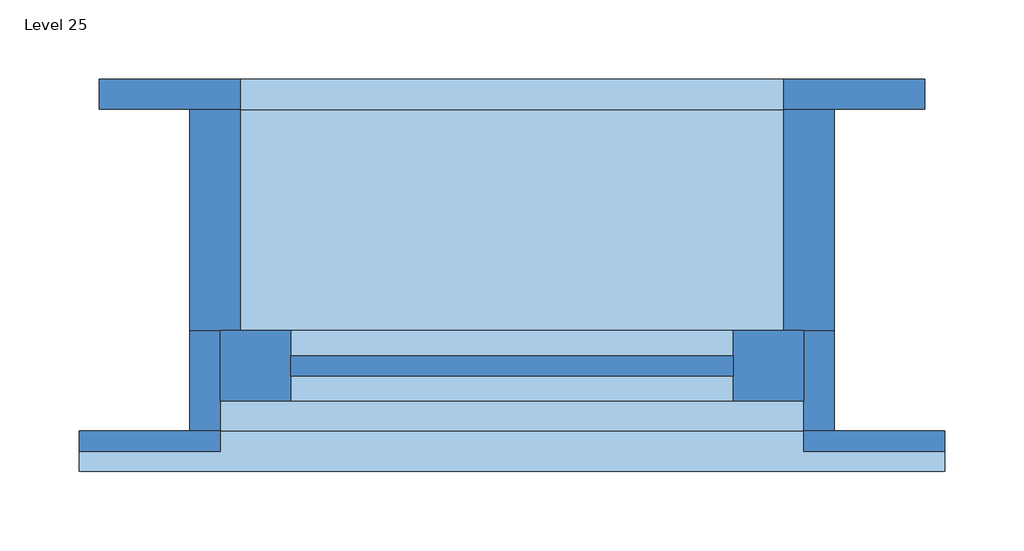
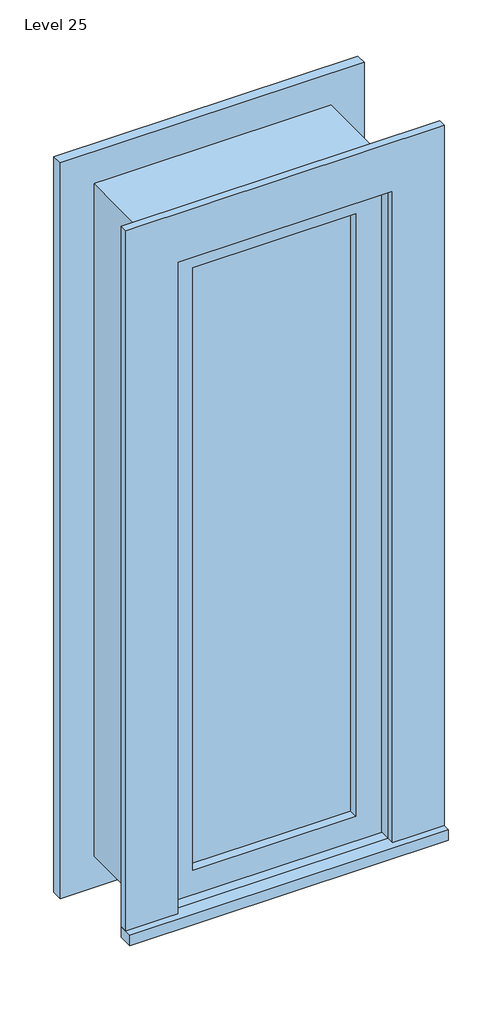
# One storey: 1 window.
"""IFC4 building model written with IfcOpenShell, lengths in millimetres."""

from ifc_helpers import new_model, si_unit, origin, place, context, project, spatial, transform, mapped, element, save
from components import window_a765b88f

model = new_model("IFC4")

# Units and contexts
model_context = context("Model", 3, world=origin())
ifc_project = project(units=[si_unit("LENGTHUNIT", "METRE", prefix="MILLI")], contexts=[model_context])

# Site, building, storey
site = spatial("IfcSite", under=ifc_project)
building = spatial("IfcBuilding", under=site)
storey = spatial("IfcBuildingStorey", under=building, Name="Level 25", Elevation=42976.8)

# Window
placement = place(None, origin())
window_shape = window_a765b88f(model_context)
element("IfcWindow", 1, ObjectType="Awning with Trim : 16\" x 48\"", at=placement, inside=storey, context=model_context, shape_type="MappedRepresentation", body=[
    mapped(window_shape, transform((20511.414721, -12354.7237084, 42976.8), x_axis=(-1.0, 0.0, 0.0), y_axis=(0.0, -1.0, 0.0), z_axis=(0.0, 0.0, 1.0))),
])

save(model, "model.ifc")

# Revit data of these elements
# Type "Awning with Trim : 16\" x 48\""
#   Type Mark = "14"
#   Construction Type Id = "GSP4R"
#   Assembly Code = "B2020100"
#   Analytic Construction = "1/8 in Pilkington single glazing"
#   Visual Light Transmittance = 0.9
#   Solar Heat Gain Coefficient = 0.78
#   Heat Transfer Coefficient (U) = 0.6496 BTU/(h·ft²·°F)
#   Height = 4' - 0"
#   Default Sill Height = 3' - 0"
#   Trim Projection - Ext. = 0' - 0 1/2"
#   Trim Projection - Int. = 0' - 0 3/4"
#   Trim Width - Exterior = 0' - 3 1/2"
#   Trim Width - Interior = 0' - 3 1/2"
#   Width = 1' - 4"
#   Window Inset = 0' - 0 3/4"
#   Define Thermal Properties by = 1
#   Glass Pane Material = Glass
#   Sash Material = Sash
#   Trim Exterior Material = Trim
#   Trim Interior Material = Trim
#   Wall Closure = (empty or 0)
# Element 1 (IfcWindow, "Awning with Trim : 16\" x 48\"")
#   Mark = "55"
#   Phase Created = New Construction
#   Materials on its faces: "Sash", "Trim", "Glass"
# Materials
#   "Glass": class "Glass", colour RGB 0 128 192, transparency 0.75, Description = "Soda Lime Glass", Cost = 0
#   "Sash": class "Wood", colour RGB 224 178 126, transparency 0
#   "Trim": class "Wood", colour RGB 224 178 126, transparency 0
